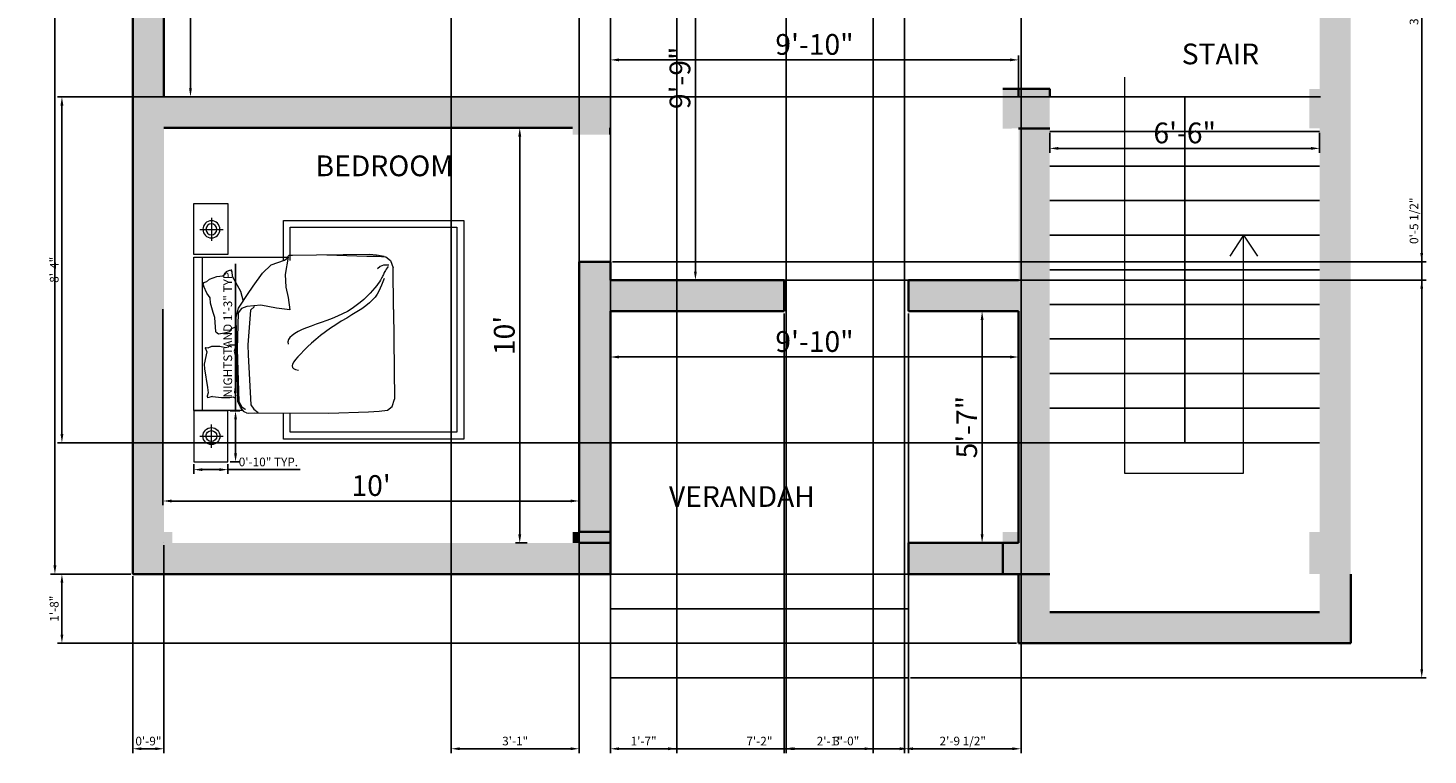
# Model space of a CAD drawing. Units: inches. Extents: x 3025 to 3429, y 1771 to 2198.
# Tile 1 of 3: x 3025 to 3429, y 1771 to 1981. Entities that reach past the tile are written whole.
import ezdxf

# ---------------------------------------------------------------- set-up
doc = ezdxf.new("R2010")
doc.units = ezdxf.units.IN
for name, color, linetype, lineweight in [('A-ANNO-DIMS', 2, 'Continuous', 18), ('A-ANNO-SYMB', 7, 'Continuous', 18), ('A-AREA-IDEN', 7, 'Continuous', 25), ('A-COLS', 7, 'Continuous', 35), ('A-FLOR-STRS', 7, 'Continuous', 25), ('A-FURN', 8, 'Continuous', 18), ('A-WALL', 7, 'Continuous', 35), ('A-WALL-PATT', 3, 'Continuous', 13)]:
    doc.layers.add(name, color=color, linetype=linetype, lineweight=lineweight)
doc.layers.add('A-COLS-PATT', color=18, linetype='Continuous', lineweight=13, true_color=0x000000)
doc.styles.get("Standard").update_dxf_attribs({"font": 'arial.ttf'})
doc.dimstyles.new('ISO-25', dxfattribs={"dimtxt": 2.5, "dimasz": 2.5, "dimexe": 1.25, "dimexo": 0.625, "dimtad": 1, "dimdec": 0, "dimlunit": 3, "dimtxsty": 'Standard', "dimcen": 2.5, "dimadec": 0, "dimazin": 0, "dimtfac": 1, "dimtdec": 0, "dimtmove": 0, "dimatfit": 3, "dimfxl": 1, "dimarcsym": 0})

# ---------------------------------------------------------------- blocks, each defined once
blk = doc.blocks.new('*D2')
at = {"layer": 'A-ANNO-DIMS', "color": 0, "lineweight": -2, "transparency": 16777216}
for p, q in [((3071.28, 2025.21), (3072.84, 2025.21)), ((3071.59, 2022.71), (3071.59, 1963.71)), ((3071.28, 1961.21), (3072.84, 1961.21))]:
    blk.add_line(p, q, dxfattribs=at)
at = {"layer": 'A-ANNO-DIMS', "color": 0, "transparency": 16777216}
for points in [[(3071.17, 2022.71), (3072, 2022.71), (3071.59, 2025.21)], [(3071.17, 1963.71), (3072, 1963.71), (3071.59, 1961.21)]]:
    blk.add_solid(points, dxfattribs=at)
at = {"layer": 'Defpoints', "color": 0, "transparency": 16777216}
for p in [(3070.66, 2025.21), (3070.66, 1961.21), (3071.59, 1961.21)]:
    blk.add_point(p, dxfattribs=at)
at = {"layer": 'A-ANNO-DIMS', "color": 0, "transparency": 16777216, "insert": (3067.91, 1993.21), "char_height": 6, "attachment_point": 5, "rotation": 90}
blk.add_mtext('5\'-4"', dxfattribs=at)
blk = doc.blocks.new('*D4')
at = {"layer": 'A-ANNO-DIMS', "color": 0, "lineweight": -2, "transparency": 16777216}
for p, q in [((3166.97, 1952.21), (3168, 1952.21)), ((3166.75, 1949.71), (3166.75, 1834.71)), ((3168.93, 1832.21), (3165.5, 1832.21))]:
    blk.add_line(p, q, dxfattribs=at)
at = {"layer": 'A-ANNO-DIMS', "color": 0, "transparency": 16777216}
for points in [[(3166.33, 1949.71), (3167.17, 1949.71), (3166.75, 1952.21)], [(3166.33, 1834.71), (3167.17, 1834.71), (3166.75, 1832.21)]]:
    blk.add_solid(points, dxfattribs=at)
at = {"layer": 'Defpoints', "color": 0, "transparency": 16777216}
for p in [(3166.35, 1952.21), (3166.75, 1832.21), (3169.56, 1832.21)]:
    blk.add_point(p, dxfattribs=at)
at = {"layer": 'A-ANNO-DIMS', "color": 0, "transparency": 16777216, "insert": (3163.06, 1892.21), "char_height": 6, "attachment_point": 5, "rotation": 90}
blk.add_mtext("10'", dxfattribs=at)
blk = doc.blocks.new('*D5')
at = {"layer": 'A-ANNO-DIMS', "color": 0, "lineweight": -2, "transparency": 16777216}
for p, q in [((3305.7, 1899.21), (3299.12, 1899.21)), ((3300.37, 1896.71), (3300.37, 1834.71)), ((3305.7, 1832.21), (3299.12, 1832.21))]:
    blk.add_line(p, q, dxfattribs=at)
at = {"layer": 'A-ANNO-DIMS', "color": 0, "transparency": 16777216}
for points in [[(3299.96, 1896.71), (3300.79, 1896.71), (3300.37, 1899.21)], [(3299.96, 1834.71), (3300.79, 1834.71), (3300.37, 1832.21)]]:
    blk.add_solid(points, dxfattribs=at)
at = {"layer": 'Defpoints', "color": 0, "transparency": 16777216}
for p in [(3306.32, 1899.21), (3300.37, 1832.21), (3306.32, 1832.21)]:
    blk.add_point(p, dxfattribs=at)
at = {"layer": 'A-ANNO-DIMS', "color": 0, "transparency": 16777216, "insert": (3296.7, 1865.71), "char_height": 6, "attachment_point": 5, "rotation": 90}
blk.add_mtext('5\'-7"', dxfattribs=at)
blk = doc.blocks.new('*D11')
at = {"layer": 'A-ANNO-DIMS', "color": 0, "lineweight": -2, "transparency": 16777216}
for p, q in [((3192.93, 1961.84), (3192.93, 1973.15)), ((3195.43, 1971.9), (3308.43, 1971.9)), ((3310.93, 1961.84), (3310.93, 1973.15))]:
    blk.add_line(p, q, dxfattribs=at)
at = {"layer": 'A-ANNO-DIMS', "color": 0, "transparency": 16777216}
for points in [[(3195.43, 1972.32), (3195.43, 1971.49), (3192.93, 1971.9)], [(3308.43, 1972.32), (3308.43, 1971.49), (3310.93, 1971.9)]]:
    blk.add_solid(points, dxfattribs=at)
at = {"layer": 'Defpoints', "color": 0, "transparency": 16777216}
for p in [(3310.93, 1971.9), (3192.93, 1961.21), (3310.93, 1961.21)]:
    blk.add_point(p, dxfattribs=at)
at = {"layer": 'A-ANNO-DIMS', "color": 0, "transparency": 16777216, "insert": (3251.93, 1975.59), "char_height": 6, "attachment_point": 5}
blk.add_mtext('9\'-10"', dxfattribs=at)
blk = doc.blocks.new('*D12')
at = {"layer": 'A-ANNO-DIMS', "color": 0, "lineweight": -2, "transparency": 16777216}
for p, q in [((3054.31, 2180.21), (3031.16, 2180.21)), ((3032.41, 2177.71), (3032.41, 1825.71)), ((3054.31, 1823.21), (3031.16, 1823.21))]:
    blk.add_line(p, q, dxfattribs=at)
at = {"layer": 'A-ANNO-DIMS', "color": 0, "transparency": 16777216}
for points in [[(3031.99, 2177.71), (3032.82, 2177.71), (3032.41, 2180.21)], [(3031.99, 1825.71), (3032.82, 1825.71), (3032.41, 1823.21)]]:
    blk.add_solid(points, dxfattribs=at)
at = {"layer": 'Defpoints', "color": 0, "transparency": 16777216}
for p in [(3054.93, 2180.21), (3032.41, 1823.21), (3054.93, 1823.21)]:
    blk.add_point(p, dxfattribs=at)
at = {"layer": 'A-ANNO-DIMS', "color": 0, "transparency": 16777216, "insert": (3028.72, 2001.71), "char_height": 6, "attachment_point": 5, "rotation": 90}
blk.add_mtext('29\'-9"', dxfattribs=at)
blk = doc.blocks.new('*D16')
at = {"layer": 'A-ANNO-DIMS', "color": 0, "lineweight": -2, "transparency": 16777216}
for p, q in [((3319.93, 1950.78), (3319.93, 1945.06)), ((3397.93, 1950.78), (3397.93, 1945.06)), ((3322.43, 1946.31), (3395.43, 1946.31))]:
    blk.add_line(p, q, dxfattribs=at)
at = {"layer": 'A-ANNO-DIMS', "color": 0, "transparency": 16777216}
for points in [[(3322.43, 1946.73), (3322.43, 1945.89), (3319.93, 1946.31)], [(3395.43, 1946.73), (3395.43, 1945.89), (3397.93, 1946.31)]]:
    blk.add_solid(points, dxfattribs=at)
at = {"layer": 'Defpoints', "color": 0, "transparency": 16777216}
for p in [(3319.93, 1951.41), (3397.93, 1951.41), (3397.93, 1946.31)]:
    blk.add_point(p, dxfattribs=at)
at = {"layer": 'A-ANNO-DIMS', "color": 0, "transparency": 16777216, "insert": (3358.93, 1950), "char_height": 6, "attachment_point": 5}
blk.add_mtext('6\'-6"', dxfattribs=at)
blk = doc.blocks.new('*D17')
at = {"layer": 'A-ANNO-DIMS', "color": 0, "lineweight": -2, "transparency": 16777216}
for p, q in [((3225.75, 2025.21), (3216.27, 2025.21)), ((3217.52, 2022.71), (3217.52, 1910.71)), ((3225.75, 1908.21), (3216.27, 1908.21))]:
    blk.add_line(p, q, dxfattribs=at)
at = {"layer": 'A-ANNO-DIMS', "color": 0, "transparency": 16777216}
for points in [[(3217.1, 2022.71), (3217.94, 2022.71), (3217.52, 2025.21)], [(3217.1, 1910.71), (3217.94, 1910.71), (3217.52, 1908.21)]]:
    blk.add_solid(points, dxfattribs=at)
at = {"layer": 'Defpoints', "color": 0, "transparency": 16777216}
for p in [(3226.37, 2025.21), (3217.52, 1908.21), (3226.37, 1908.21)]:
    blk.add_point(p, dxfattribs=at)
at = {"layer": 'A-ANNO-DIMS', "color": 0, "transparency": 16777216, "insert": (3213.83, 1966.71), "char_height": 6, "attachment_point": 5, "rotation": 90}
blk.add_mtext('9\'-9"', dxfattribs=at)
blk = doc.blocks.new('*D18')
at = {"layer": 'A-ANNO-DIMS', "color": 0, "lineweight": -2, "transparency": 16777216}
for p, q in [((3192.93, 1865.6), (3192.93, 1887.24)), ((3195.43, 1885.99), (3308.43, 1885.99)), ((3310.93, 1865.6), (3310.93, 1887.24))]:
    blk.add_line(p, q, dxfattribs=at)
at = {"layer": 'A-ANNO-DIMS', "color": 0, "transparency": 16777216}
for points in [[(3195.43, 1886.4), (3195.43, 1885.57), (3192.93, 1885.99)], [(3308.43, 1886.4), (3308.43, 1885.57), (3310.93, 1885.99)]]:
    blk.add_solid(points, dxfattribs=at)
at = {"layer": 'Defpoints', "color": 0, "transparency": 16777216}
for p in [(3310.93, 1885.99), (3192.93, 1864.97), (3310.93, 1864.97)]:
    blk.add_point(p, dxfattribs=at)
at = {"layer": 'A-ANNO-DIMS', "color": 0, "transparency": 16777216, "insert": (3251.93, 1889.68), "char_height": 6, "attachment_point": 5}
blk.add_mtext('9\'-10"', dxfattribs=at)
blk = doc.blocks.new('*D19')
at = {"layer": 'A-ANNO-DIMS', "color": 0, "lineweight": -2, "transparency": 16777216}
for p, q in [((3063.64, 1899.86), (3063.64, 1843.1)), ((3183.93, 1899.86), (3183.93, 1843.1)), ((3181.43, 1844.35), (3066.14, 1844.35))]:
    blk.add_line(p, q, dxfattribs=at)
at = {"layer": 'A-ANNO-DIMS', "color": 0, "transparency": 16777216}
for points in [[(3066.14, 1844.77), (3066.14, 1843.94), (3063.64, 1844.35)], [(3181.43, 1844.77), (3181.43, 1843.94), (3183.93, 1844.35)]]:
    blk.add_solid(points, dxfattribs=at)
at = {"layer": 'Defpoints', "color": 0, "transparency": 16777216}
for p in [(3063.64, 1900.48), (3183.93, 1900.48), (3063.64, 1844.35)]:
    blk.add_point(p, dxfattribs=at)
at = {"layer": 'A-ANNO-DIMS', "color": 0, "transparency": 16777216, "insert": (3123.79, 1848.04), "char_height": 6, "attachment_point": 5}
blk.add_mtext("10'", dxfattribs=at)
blk = doc.blocks.new('NIGHTSTAND-15IN')
for p, q in [((5.1, 4.12), (5.1, 10.82)), ((1.74, 7.47), (8.45, 7.47))]:
    blk.add_line(p, q)
blk.add_lwpolyline([(9.86, 0), (9.86, 14.79), (0, 14.79), (0, 0)], close=True)
for radius in [2.47, 1.58]:
    blk.add_circle((5.1, 7.47), radius)
blk = doc.blocks.new('*D27')
at = {"layer": 'A-ANNO-DIMS', "color": 0, "lineweight": -2, "transparency": 16777216}
for p, q in [((3084.61, 1870.42), (3084.61, 1912.96)), ((3083.02, 1870.42), (3085.86, 1870.42)), ((3084.61, 1858.14), (3084.61, 1867.92)), ((3083.02, 1855.64), (3085.86, 1855.64))]:
    blk.add_line(p, q, dxfattribs=at)
at = {"layer": 'A-ANNO-DIMS', "color": 0, "transparency": 16777216}
for points in [[(3084.2, 1867.92), (3085.03, 1867.92), (3084.61, 1870.42)], [(3084.2, 1858.14), (3085.03, 1858.14), (3084.61, 1855.64)]]:
    blk.add_solid(points, dxfattribs=at)
at = {"layer": 'Defpoints', "color": 0, "transparency": 16777216}
for p in [(3082.39, 1870.42), (3084.61, 1870.42), (3082.39, 1855.64)]:
    blk.add_point(p, dxfattribs=at)
at = {"layer": 'A-ANNO-DIMS', "color": 0, "transparency": 16777216, "insert": (3082.69, 1892.94), "char_height": 2.5, "attachment_point": 5, "rotation": 90}
blk.add_mtext('NIGHTSTAND 1\'-3" TYP.', dxfattribs=at)
blk = doc.blocks.new('*D28')
at = {"layer": 'A-ANNO-DIMS', "color": 0, "lineweight": -2, "transparency": 16777216}
for p, q in [((3072.54, 1855.01), (3072.54, 1852.17)), ((3075.04, 1853.42), (3079.89, 1853.42)), ((3082.39, 1855.01), (3082.39, 1852.17)), ((3082.39, 1853.42), (3103.33, 1853.42))]:
    blk.add_line(p, q, dxfattribs=at)
at = {"layer": 'A-ANNO-DIMS', "color": 0, "transparency": 16777216}
for points in [[(3075.04, 1853.84), (3075.04, 1853), (3072.54, 1853.42)], [(3079.89, 1853.84), (3079.89, 1853), (3082.39, 1853.42)]]:
    blk.add_solid(points, dxfattribs=at)
at = {"layer": 'Defpoints', "color": 0, "transparency": 16777216}
for p in [(3072.54, 1855.64), (3082.39, 1855.64), (3082.39, 1853.42)]:
    blk.add_point(p, dxfattribs=at)
at = {"layer": 'A-ANNO-DIMS', "color": 0, "transparency": 16777216, "insert": (3094.11, 1855.32), "char_height": 2.5, "attachment_point": 5}
blk.add_mtext('0\'-10" TYP.', dxfattribs=at)
blk = doc.blocks.new('*D29')
at = {"layer": 'A-ANNO-DIMS', "color": 0, "lineweight": -2, "transparency": 16777216}
for p, q in [((3407.56, 2180.21), (3428.68, 2180.21)), ((3427.43, 2177.71), (3427.43, 1795.71)), ((3279.71, 1793.21), (3428.68, 1793.21))]:
    blk.add_line(p, q, dxfattribs=at)
at = {"layer": 'A-ANNO-DIMS', "color": 0, "transparency": 16777216}
for points in [[(3427.02, 2177.71), (3427.85, 2177.71), (3427.43, 2180.21)], [(3427.02, 1795.71), (3427.85, 1795.71), (3427.43, 1793.21)]]:
    blk.add_solid(points, dxfattribs=at)
at = {"layer": 'Defpoints', "color": 0, "transparency": 16777216}
for p in [(3406.93, 2180.21), (3279.09, 1793.21), (3427.43, 1793.21)]:
    blk.add_point(p, dxfattribs=at)
at = {"layer": 'A-ANNO-DIMS', "color": 0, "transparency": 16777216, "insert": (3425.53, 1986.71), "char_height": 2.5, "attachment_point": 5, "rotation": 90}
blk.add_mtext('32\'-3"', dxfattribs=at)
blk = doc.blocks.new('*D30')
at = {"layer": 'A-ANNO-DIMS', "color": 0, "lineweight": -2, "transparency": 16777216}
for p, q in [((3192.93, 1792.59), (3192.93, 1771.46)), ((3279.09, 1792.59), (3279.09, 1771.46)), ((3195.43, 1772.71), (3276.59, 1772.71))]:
    blk.add_line(p, q, dxfattribs=at)
at = {"layer": 'A-ANNO-DIMS', "color": 0, "transparency": 16777216}
for points in [[(3195.43, 1773.13), (3195.43, 1772.3), (3192.93, 1772.71)], [(3276.59, 1773.13), (3276.59, 1772.3), (3279.09, 1772.71)]]:
    blk.add_solid(points, dxfattribs=at)
at = {"layer": 'Defpoints', "color": 0, "transparency": 16777216}
for p in [(3192.93, 1793.21), (3279.09, 1793.21), (3279.09, 1772.71)]:
    blk.add_point(p, dxfattribs=at)
at = {"layer": 'A-ANNO-DIMS', "color": 0, "transparency": 16777216, "insert": (3236.01, 1774.59), "char_height": 2.5, "attachment_point": 5}
blk.add_mtext('7\'-2"', dxfattribs=at)
blk = doc.blocks.new('*D31')
at = {"layer": 'A-ANNO-DIMS', "color": 0, "lineweight": -2, "transparency": 16777216}
for p, q in [((3243.14, 1898.59), (3243.14, 1771.46)), ((3279.09, 1898.59), (3279.09, 1771.46)), ((3245.64, 1772.71), (3276.59, 1772.71))]:
    blk.add_line(p, q, dxfattribs=at)
at = {"layer": 'A-ANNO-DIMS', "color": 0, "transparency": 16777216}
for points in [[(3245.64, 1773.13), (3245.64, 1772.3), (3243.14, 1772.71)], [(3276.59, 1773.13), (3276.59, 1772.3), (3279.09, 1772.71)]]:
    blk.add_solid(points, dxfattribs=at)
at = {"layer": 'Defpoints', "color": 0, "transparency": 16777216}
for p in [(3243.14, 1899.21), (3279.09, 1899.21), (3279.09, 1772.71)]:
    blk.add_point(p, dxfattribs=at)
at = {"layer": 'A-ANNO-DIMS', "color": 0, "transparency": 16777216, "insert": (3261.11, 1774.62), "char_height": 2.5, "attachment_point": 5}
blk.add_mtext('3\'-0"', dxfattribs=at)
blk = doc.blocks.new('*D32')
at = {"layer": 'A-ANNO-DIMS', "color": 0, "lineweight": -2, "transparency": 16777216}
for p, q in [((3063.93, 1831.59), (3063.93, 1771.46)), ((3054.93, 1822.59), (3054.93, 1771.46)), ((3057.43, 1772.71), (3061.43, 1772.71))]:
    blk.add_line(p, q, dxfattribs=at)
at = {"layer": 'A-ANNO-DIMS', "color": 0, "transparency": 16777216}
for points in [[(3057.43, 1773.13), (3057.43, 1772.3), (3054.93, 1772.71)], [(3061.43, 1773.13), (3061.43, 1772.3), (3063.93, 1772.71)]]:
    blk.add_solid(points, dxfattribs=at)
at = {"layer": 'Defpoints', "color": 0, "transparency": 16777216}
for p in [(3063.93, 1832.21), (3054.93, 1823.21), (3063.93, 1772.71)]:
    blk.add_point(p, dxfattribs=at)
at = {"layer": 'A-ANNO-DIMS', "color": 0, "transparency": 16777216, "insert": (3059.43, 1774.61), "char_height": 2.5, "attachment_point": 5}
blk.add_mtext('0\'-9"', dxfattribs=at)
blk = doc.blocks.new('*D33')
at = {"layer": 'A-ANNO-DIMS', "color": 0, "lineweight": -2, "transparency": 16777216}
for p, q in [((3054.31, 1823.21), (3033.18, 1823.21)), ((3034.43, 1820.71), (3034.43, 1805.71)), ((3310.31, 1803.21), (3033.18, 1803.21))]:
    blk.add_line(p, q, dxfattribs=at)
at = {"layer": 'A-ANNO-DIMS', "color": 0, "transparency": 16777216}
for points in [[(3034.02, 1820.71), (3034.85, 1820.71), (3034.43, 1823.21)], [(3034.02, 1805.71), (3034.85, 1805.71), (3034.43, 1803.21)]]:
    blk.add_solid(points, dxfattribs=at)
at = {"layer": 'Defpoints', "color": 0, "transparency": 16777216}
for p in [(3054.93, 1823.21), (3034.43, 1803.21), (3310.93, 1803.21)]:
    blk.add_point(p, dxfattribs=at)
at = {"layer": 'A-ANNO-DIMS', "color": 0, "transparency": 16777216, "insert": (3032.53, 1813.21), "char_height": 2.5, "attachment_point": 5, "rotation": 90}
blk.add_mtext('1\'-8"', dxfattribs=at)
blk = doc.blocks.new('*D34')
at = {"layer": 'A-ANNO-DIMS', "color": 0, "lineweight": -2, "transparency": 16777216}
for p, q in [((3358.31, 1961.21), (3033.18, 1961.21)), ((3034.43, 1958.71), (3034.43, 1863.71)), ((3358.31, 1861.21), (3033.18, 1861.21))]:
    blk.add_line(p, q, dxfattribs=at)
at = {"layer": 'A-ANNO-DIMS', "color": 0, "transparency": 16777216}
for points in [[(3034.02, 1958.71), (3034.85, 1958.71), (3034.43, 1961.21)], [(3034.02, 1863.71), (3034.85, 1863.71), (3034.43, 1861.21)]]:
    blk.add_solid(points, dxfattribs=at)
at = {"layer": 'Defpoints', "color": 0, "transparency": 16777216}
for p in [(3358.93, 1961.21), (3034.43, 1861.21), (3358.93, 1861.21)]:
    blk.add_point(p, dxfattribs=at)
at = {"layer": 'A-ANNO-DIMS', "color": 0, "transparency": 16777216, "insert": (3032.53, 1911.21), "char_height": 2.5, "attachment_point": 5, "rotation": 90}
blk.add_mtext('8\'-4"', dxfattribs=at)
blk = doc.blocks.new('*D35')
at = {"layer": 'A-ANNO-DIMS', "color": 0, "lineweight": -2, "transparency": 16777216}
for p, q in [((3268.93, 2036.1), (3268.93, 1771.46)), ((3243.74, 2033.59), (3243.74, 1771.46)), ((3246.24, 1772.71), (3266.43, 1772.71))]:
    blk.add_line(p, q, dxfattribs=at)
at = {"layer": 'A-ANNO-DIMS', "color": 0, "transparency": 16777216}
for points in [[(3246.24, 1773.13), (3246.24, 1772.3), (3243.74, 1772.71)], [(3266.43, 1773.13), (3266.43, 1772.3), (3268.93, 1772.71)]]:
    blk.add_solid(points, dxfattribs=at)
at = {"layer": 'Defpoints', "color": 0, "transparency": 16777216}
for p in [(3268.93, 2036.73), (3243.74, 2034.21), (3268.93, 1772.71)]:
    blk.add_point(p, dxfattribs=at)
at = {"layer": 'A-ANNO-DIMS', "color": 0, "transparency": 16777216, "insert": (3256.34, 1774.59), "char_height": 2.5, "attachment_point": 5}
blk.add_mtext('2\'-1"', dxfattribs=at)
blk = doc.blocks.new('*D36')
at = {"layer": 'A-ANNO-DIMS', "color": 0, "lineweight": -2, "transparency": 16777216}
for p, q in [((3277.93, 2036.1), (3277.93, 1771.46)), ((3311.62, 2033.59), (3311.62, 1771.46)), ((3280.43, 1772.71), (3309.12, 1772.71))]:
    blk.add_line(p, q, dxfattribs=at)
at = {"layer": 'A-ANNO-DIMS', "color": 0, "transparency": 16777216}
for points in [[(3280.43, 1773.13), (3280.43, 1772.3), (3277.93, 1772.71)], [(3309.12, 1773.13), (3309.12, 1772.3), (3311.62, 1772.71)]]:
    blk.add_solid(points, dxfattribs=at)
at = {"layer": 'Defpoints', "color": 0, "transparency": 16777216}
for p in [(3277.93, 2036.73), (3311.62, 2034.21), (3311.62, 1772.71)]:
    blk.add_point(p, dxfattribs=at)
at = {"layer": 'A-ANNO-DIMS', "color": 0, "transparency": 16777216, "insert": (3294.78, 1774.63), "char_height": 2.5, "attachment_point": 5}
blk.add_mtext('2\'-9 1/2"', dxfattribs=at)
blk = doc.blocks.new('*D37')
at = {"layer": 'A-ANNO-DIMS', "color": 0, "lineweight": -2, "transparency": 16777216}
for p, q in [((3183.93, 2035.84), (3183.93, 1771.46)), ((3146.93, 2033.59), (3146.93, 1771.46)), ((3149.43, 1772.71), (3181.43, 1772.71))]:
    blk.add_line(p, q, dxfattribs=at)
at = {"layer": 'A-ANNO-DIMS', "color": 0, "transparency": 16777216}
for points in [[(3149.43, 1773.13), (3149.43, 1772.3), (3146.93, 1772.71)], [(3181.43, 1773.13), (3181.43, 1772.3), (3183.93, 1772.71)]]:
    blk.add_solid(points, dxfattribs=at)
at = {"layer": 'Defpoints', "color": 0, "transparency": 16777216}
for p in [(3183.93, 2036.47), (3146.93, 2034.21), (3183.93, 1772.71)]:
    blk.add_point(p, dxfattribs=at)
at = {"layer": 'A-ANNO-DIMS', "color": 0, "transparency": 16777216, "insert": (3165.43, 1774.62), "char_height": 2.5, "attachment_point": 5}
blk.add_mtext('3\'-1"', dxfattribs=at)
blk = doc.blocks.new('*D38')
at = {"layer": 'A-ANNO-DIMS', "color": 0, "lineweight": -2, "transparency": 16777216}
for p, q in [((3427.43, 1916.03), (3427.43, 1932.25)), ((3193.56, 1913.53), (3428.68, 1913.53)), ((3427.43, 1908.21), (3427.43, 1913.53)), ((3193.56, 1908.21), (3428.68, 1908.21)), ((3427.43, 1905.71), (3427.43, 1903.21))]:
    blk.add_line(p, q, dxfattribs=at)
at = {"layer": 'A-ANNO-DIMS', "color": 0, "transparency": 16777216}
for points in [[(3427.02, 1916.03), (3427.85, 1916.03), (3427.43, 1913.53)], [(3427.02, 1905.71), (3427.85, 1905.71), (3427.43, 1908.21)]]:
    blk.add_solid(points, dxfattribs=at)
at = {"layer": 'Defpoints', "color": 0, "transparency": 16777216}
for p in [(3192.93, 1913.53), (3427.43, 1913.53), (3192.93, 1908.21)]:
    blk.add_point(p, dxfattribs=at)
at = {"layer": 'A-ANNO-DIMS', "color": 0, "transparency": 16777216, "insert": (3425.52, 1925.39), "char_height": 2.5, "attachment_point": 5, "rotation": 90}
blk.add_mtext('0\'-5 1/2"', dxfattribs=at)
blk = doc.blocks.new('*D40')
at = {"layer": 'A-ANNO-DIMS', "color": 0, "lineweight": -2, "transparency": 16777216}
for p, q in [((3192.93, 2033.59), (3192.93, 1771.46)), ((3212.14, 2033.59), (3212.14, 1771.46)), ((3195.43, 1772.71), (3209.64, 1772.71))]:
    blk.add_line(p, q, dxfattribs=at)
at = {"layer": 'A-ANNO-DIMS', "color": 0, "transparency": 16777216}
for points in [[(3195.43, 1773.13), (3195.43, 1772.3), (3192.93, 1772.71)], [(3209.64, 1773.13), (3209.64, 1772.3), (3212.14, 1772.71)]]:
    blk.add_solid(points, dxfattribs=at)
at = {"layer": 'Defpoints', "color": 0, "transparency": 16777216}
for p in [(3192.93, 2034.21), (3212.14, 2034.21), (3212.14, 1772.71)]:
    blk.add_point(p, dxfattribs=at)
at = {"layer": 'A-ANNO-DIMS', "color": 0, "transparency": 16777216, "insert": (3202.54, 1774.59), "char_height": 2.5, "attachment_point": 5}
blk.add_mtext('1\'-7"', dxfattribs=at)

msp = doc.modelspace()

# ---------------------------------------------------------------- hatches: boundary and pattern name
at = {"layer": 'A-COLS-PATT'}
h = msp.add_hatch(color=256, dxfattribs=at)
h.dxf.hatch_style = 1
h.paths.add_polyline_path([(3310.93, 1835.41), (3306.32, 1835.41), (3306.32, 1832.21), (3310.93, 1832.21)], flags=17)
h.paths.add_polyline_path([(3319.93, 1832.21), (3319.93, 1835.41), (3310.93, 1835.41), (3310.93, 1832.21), (3306.32, 1832.21), (3306.32, 1823.21), (3310.93, 1823.21), (3319.93, 1823.21)])
h.paths.add_polyline_path([(3310.93, 1961.21), (3310.93, 1963.51), (3306.32, 1963.51), (3306.32, 1952.02), (3310.93, 1952.09)])
h.paths.add_polyline_path([(3319.93, 1961.21), (3310.93, 1961.21), (3310.93, 1952.09), (3319.93, 1952.09)])
h = msp.add_hatch(color=256, dxfattribs=at)
h.dxf.hatch_style = 1
h.paths.add_polyline_path([(3397.93, 1963.51), (3394.99, 1963.51), (3394.99, 1961.21), (3397.93, 1961.21)])
h.paths.add_polyline_path([(3319.94, 1963.51), (3310.93, 1963.51), (3310.93, 1961.21), (3319.94, 1961.21)])
h.paths.add_polyline_path([(3397.93, 1961.21), (3394.99, 1961.21), (3394.99, 1952.09), (3397.93, 1952.09)])
h.paths.add_polyline_path([(3406.93, 1963.51), (3397.93, 1963.51), (3397.93, 1952.09), (3406.93, 1952.09)])
h.paths.add_polyline_path([(3397.93, 1832.21), (3397.93, 1835.41), (3394.99, 1835.41), (3394.99, 1823.21), (3397.93, 1823.21)])
h.paths.add_polyline_path([(3406.93, 1835.41), (3397.93, 1835.41), (3397.93, 1832.21), (3397.93, 1823.21), (3406.93, 1823.21)])
h = msp.add_hatch(color=256, dxfattribs=at)
h.dxf.hatch_style = 1
h.paths.add_polyline_path([(3192.93, 1961.21), (3182.07, 1961.21), (3182.07, 1952.21), (3192.93, 1952.21)])
h = msp.add_hatch(color=256, dxfattribs=at)
h.dxf.hatch_style = 1
h.paths.add_polyline_path([(3192.87, 1952.21), (3182.07, 1952.21), (3182.07, 1950.3), (3192.87, 1950.3)])
h = msp.add_hatch(color=256, dxfattribs=at)
h.dxf.hatch_style = 1
h.paths.add_polyline_path([(3066.3, 1832.21), (3063.93, 1832.21), (3063.93, 1835.41), (3054.93, 1835.41), (3054.93, 1823.21), (3066.3, 1823.21)])
h.paths.add_polyline_path([(3066.3, 1835.41), (3063.93, 1835.41), (3063.93, 1832.21), (3066.3, 1832.21)], flags=17)
h = msp.add_hatch(color=256, dxfattribs=at)
h.dxf.hatch_style = 1
h.paths.add_polyline_path([(3183.93, 1835.41), (3182.07, 1835.41), (3182.07, 1832.21), (3183.93, 1832.21)])
h = msp.add_hatch(color=256, dxfattribs=at)
h.dxf.hatch_style = 1
h.paths.add_polyline_path([(3192.93, 1835.41), (3183.93, 1835.41), (3183.93, 1832.21), (3192.93, 1832.21)])
h = msp.add_hatch(color=256, dxfattribs=at)
h.dxf.hatch_style = 1
h.paths.add_polyline_path([(3192.93, 1832.21), (3183.93, 1832.21), (3182.07, 1832.21), (3182.07, 1823.21), (3192.93, 1823.21)])
at = {"layer": 'A-WALL-PATT'}
h = msp.add_hatch(color=256, dxfattribs=at)
h.dxf.hatch_style = 1
h.paths.add_polyline_path([(3063.93, 1952.21), (3192.93, 1952.21), (3192.93, 1961.21), (3063.93, 1961.21), (3063.93, 2025.21), (3054.93, 2025.21), (3054.93, 1823.21), (3192.93, 1823.21), (3192.93, 1832.21), (3183.93, 1832.21), (3063.93, 1832.21)])
h.paths.add_polyline_path([(3146.93, 2034.21), (3063.93, 2034.21), (3063.93, 2036.54), (3054.93, 2036.54), (3054.93, 2025.21), (3063.93, 2025.21), (3137.93, 2025.21), (3137.93, 1993.21), (3146.93, 1993.21)])
h.paths.add_polyline_path([(3063.93, 2167.94), (3054.93, 2167.94), (3054.93, 2036.54), (3063.93, 2036.54)])
h.paths.add_polyline_path([(3182.07, 2180.21), (3066.24, 2180.21), (3066.24, 2171.21), (3182.07, 2171.21)])
h.paths.add_polyline_path([(3192.93, 2114.21), (3243.74, 2114.21), (3243.74, 2123.21), (3192.93, 2123.21), (3192.93, 2167.95), (3183.93, 2167.95), (3183.93, 2036.47), (3192.93, 2036.47)])
h = msp.add_hatch(color=256, dxfattribs=at)
h.dxf.hatch_style = 1
h.paths.add_polyline_path([(3406.93, 1823.21), (3397.93, 1823.21), (3397.93, 1812.21), (3319.93, 1812.21), (3319.93, 1823.21), (3310.93, 1823.21), (3310.93, 1803.21), (3406.93, 1803.21)])
h.paths.add_polyline_path([(3406.93, 1952.09), (3397.93, 1952.09), (3397.93, 1835.41), (3406.93, 1835.41)])
h.paths.add_polyline_path([(3406.93, 2025.21), (3397.93, 2025.21), (3397.93, 1963.51), (3406.93, 1963.51)])
h = msp.add_hatch(color=256, dxfattribs=at)
h.dxf.hatch_style = 1
h.paths.add_polyline_path([(3306.32, 1908.21), (3279.09, 1908.21), (3279.09, 1899.21), (3306.32, 1899.21)])
h.paths.add_polyline_path([(3319.93, 1952.09), (3310.93, 1952.09), (3310.93, 1908.21), (3306.32, 1908.21), (3306.32, 1899.21), (3310.93, 1899.21), (3310.93, 1841.21), (3310.93, 1835.41), (3319.93, 1835.41)])
h = msp.add_hatch(color=256, dxfattribs=at)
h.dxf.hatch_style = 1
h.paths.add_polyline_path([(3243.14, 1899.21), (3243.14, 1908.21), (3192.93, 1908.21), (3192.93, 1913.53), (3183.93, 1913.53), (3183.93, 1835.41), (3192.93, 1835.41), (3192.93, 1899.21)])
h = msp.add_hatch(color=256, dxfattribs=at)
h.dxf.hatch_style = 1
h.paths.add_polyline_path([(3306.32, 1832.21), (3279.09, 1832.21), (3279.09, 1823.21), (3306.32, 1823.21)])

# ---------------------------------------------------------------- linework, layer by layer
at = {"layer": 'A-ANNO-SYMB'}
for p, q in [((3341.52, 1966.91), (3341.52, 1852.41)), ((3375.96, 1921.21), (3371.98, 1915.16)), ((3375.96, 1852.41), (3375.96, 1921.21)), ((3375.96, 1921.21), (3379.95, 1915.16)), ((3341.52, 1852.41), (3375.96, 1852.41))]:
    msp.add_line(p, q, dxfattribs=at)
at = {"layer": 'A-COLS'}
for p, q in [((3306.32, 1963.51), (3310.93, 1963.51)), ((3310.93, 1963.51), (3310.93, 1961.21)), ((3310.93, 1963.51), (3319.94, 1963.51)), ((3319.94, 1963.51), (3319.94, 1961.21)), ((3192.87, 1950.3), (3192.87, 1952.21)), ((3310.93, 1952.09), (3319.93, 1952.09)), ((3183.93, 1835.41), (3192.93, 1835.41)), ((3183.93, 1832.21), (3192.93, 1832.21)), ((3306.32, 1832.21), (3306.32, 1823.21)), ((3310.93, 1823.21), (3319.93, 1823.21))]:
    msp.add_line(p, q, dxfattribs=at)
at = {"layer": 'A-FLOR-STRS'}
for p, q in [((3358.93, 1961.21), (3319.94, 1961.21)), ((3358.93, 1961.21), (3358.93, 1861.21)), ((3358.93, 1961.21), (3398.16, 1961.21)), ((3319.93, 1951.21), (3397.93, 1951.21)), ((3319.93, 1941.21), (3397.93, 1941.21)), ((3319.93, 1931.21), (3397.93, 1931.21)), ((3319.93, 1921.21), (3397.93, 1921.21)), ((3319.93, 1911.21), (3397.93, 1911.21)), ((3319.93, 1901.21), (3397.93, 1901.21)), ((3319.93, 1891.21), (3397.93, 1891.21)), ((3319.93, 1881.21), (3397.93, 1881.21)), ((3319.93, 1871.21), (3397.93, 1871.21)), ((3319.93, 1861.21), (3397.93, 1861.21)), ((3192.93, 1823.21), (3279.09, 1823.21)), ((3192.93, 1823.21), (3192.93, 1813.21)), ((3279.09, 1793.21), (3279.09, 1823.21)), ((3192.93, 1813.21), (3192.93, 1803.21)), ((3192.93, 1813.21), (3279.09, 1813.21)), ((3192.93, 1803.21), (3192.93, 1793.21)), ((3192.93, 1803.21), (3279.09, 1803.21)), ((3192.93, 1793.21), (3279.09, 1793.21))]:
    msp.add_line(p, q, dxfattribs=at)
at = {"layer": 'A-FURN'}
for p, q in [((3099.76, 1914.78), (3099.72, 1914.87)), ((3108.02, 1915.44), (3101.05, 1915.37)), ((3123.28, 1915.59), (3108.02, 1915.44)), ((3111.01, 1915.49), (3122.54, 1915.19)), ((3122.54, 1915.19), (3125.56, 1915.12)), ((3125.39, 1915.47), (3123.28, 1915.59)), ((3127.59, 1915.05), (3125.39, 1915.47)), ((3125.56, 1915.12), (3128.05, 1914.92)), ((3128.05, 1914.92), (3129.39, 1913.88)), ((3129.39, 1913.88), (3130.16, 1911.8)), ((3080.93, 1909.46), (3081.59, 1909.99)), ((3081.59, 1909.99), (3082.02, 1910.68)), ((3082.02, 1910.68), (3083.11, 1911.15)), ((3083.11, 1911.15), (3083.56, 1910.57)), ((3083.56, 1910.57), (3083.61, 1909.37)), ((3126.4, 1912.19), (3125.65, 1911.47)), ((3127.42, 1912.52), (3126.4, 1912.19)), ((3128.88, 1912.59), (3127.42, 1912.52)), ((3130.16, 1906.86), (3130.16, 1911.8)), ((3076.36, 1904.45), (3075.44, 1906.41)), ((3076.21, 1907.74), (3077.07, 1908.52)), ((3077.07, 1908.52), (3079.21, 1909.27)), ((3079.21, 1909.27), (3080.93, 1909.46)), ((3083.61, 1909.37), (3086.06, 1905)), ((3130.3, 1904.99), (3130.16, 1906.86)), ((3077.28, 1903.07), (3076.36, 1904.45)), ((3077.28, 1903.07), (3076.36, 1904.45)), ((3077.41, 1901.51), (3077.28, 1903.07)), ((3130.3, 1899.7), (3130.3, 1904.99)), ((3078.13, 1898.84), (3077.41, 1901.51)), ((3078.66, 1897.43), (3078.13, 1898.84)), ((3130.3, 1899.7), (3130.58, 1873.8)), ((3078.9, 1893.26), (3078.66, 1897.43)), ((3076.28, 1887.52), (3075.52, 1883.89)), ((3075.9, 1888.75), (3075.87, 1888.64)), ((3075.87, 1888.64), (3076.28, 1887.52)), ((3075.9, 1888.75), (3076.72, 1888.66)), ((3075.9, 1888.75), (3076.72, 1888.66)), ((3076.72, 1888.66), (3077.79, 1889.11)), ((3077.79, 1889.11), (3080.06, 1889.09)), ((3080.06, 1889.09), (3081.74, 1888.69)), ((3081.74, 1888.69), (3082.54, 1888.97)), ((3082.54, 1888.97), (3083.18, 1889.46)), ((3083.18, 1889.46), (3084.37, 1889.53)), ((3084.6, 1888.84), (3084.24, 1887.7)), ((3084.24, 1887.7), (3085.15, 1884.1)), ((3084.37, 1889.53), (3084.6, 1888.84)), ((3075.52, 1883.89), (3075.67, 1882.54)), ((3077.96, 1874.56), (3076.53, 1874.18)), ((3129.88, 1871.7), (3130.58, 1873.8)), ((3086.8, 1870.48), (3072.54, 1870.48)), ((3087.78, 1869.85), (3088.47, 1869.79)), ((3088.47, 1869.79), (3090.07, 1869.81)), ((3090.07, 1869.81), (3111.55, 1869.72)), ((3111.55, 1869.72), (3123.06, 1870.18)), ((3123.06, 1870.18), (3126.08, 1870.34)), ((3126.08, 1870.34), (3128.56, 1870.62)), ((3128.56, 1870.62), (3129.88, 1871.7))]:
    msp.add_line(p, q, dxfattribs=at)
for points in [[(3098.46, 1913.9), (3098.46, 1925.5), (3150.56, 1925.5), (3150.56, 1862.24), (3098.46, 1862.24), (3098.46, 1869.78)], [(3100.43, 1913.9), (3100.43, 1923.53), (3148.59, 1923.53), (3148.59, 1864.21), (3100.43, 1864.21), (3100.43, 1869.78)], [(3072.54, 1870.48), (3072.54, 1914.85), (3099.68, 1914.85)], [(3075, 1914.85), (3075, 1870.48)], [(3086.53, 1870.85), (3086, 1871.46), (3085.31, 1873.12), (3084.83, 1897.64), (3085.46, 1900.1), (3088.07, 1904.04), (3089.71, 1906.51), (3092.44, 1910.23), (3094.86, 1912.6), (3098.74, 1914), (3099.75, 1914.69)], [(3099.78, 1914.85), (3098.91, 1909.88), (3099.19, 1906.21), (3099.79, 1903.21), (3100.29, 1899.65), (3096.41, 1900.13), (3091.89, 1900.93), (3087.9, 1900.58), (3086.29, 1900.06), (3085.37, 1898.76), (3085.08, 1888.24), (3085.53, 1873.13), (3086.45, 1871.58), (3087.35, 1870.93), (3087.43, 1870.84)], [(3100.99, 1915.37), (3100.03, 1915.3), (3099.74, 1915.02), (3099.68, 1914.85)], [(3128.72, 1912.15), (3128.41, 1911.74), (3128.15, 1911.37), (3127.94, 1911.03), (3127.76, 1910.71), (3127.61, 1910.41), (3127.48, 1910.13), (3127.35, 1909.84), (3127.22, 1909.56), (3127.09, 1909.26), (3126.93, 1908.94), (3126.74, 1908.59), (3126.5, 1908.2), (3126.2, 1907.75), (3125.84, 1907.24), (3125.4, 1906.67), (3124.86, 1906), (3124.23, 1905.26), (3123.49, 1904.44), (3122.64, 1903.57), (3121.7, 1902.66), (3120.66, 1901.75), (3119.52, 1900.86), (3118.29, 1899.99), (3116.95, 1899.18), (3115.53, 1898.43), (3114.04, 1897.75), (3112.5, 1897.13), (3110.95, 1896.54), (3109.4, 1895.99), (3107.89, 1895.47), (3106.44, 1894.95), (3105.08, 1894.43), (3103.82, 1893.91), (3102.7, 1893.37), (3101.73, 1892.82), (3100.93, 1892.25), (3100.32, 1891.66), (3099.92, 1891.05), (3099.74, 1890.41), (3099.82, 1889.73)], [(3076.21, 1907.74), (3075.31, 1907.46), (3075.12, 1906.87), (3075.44, 1906.41)], [(3127.56, 1908.65), (3127.15, 1907.71), (3126.77, 1906.79), (3126.39, 1905.9), (3125.98, 1905.03), (3125.5, 1904.17), (3124.92, 1903.32), (3124.22, 1902.48), (3123.34, 1901.63), (3122.29, 1900.79), (3121.07, 1899.93), (3119.71, 1899.06), (3118.26, 1898.17), (3116.74, 1897.26), (3115.18, 1896.31), (3113.61, 1895.33), (3112.07, 1894.32), (3110.59, 1893.26), (3109.17, 1892.17), (3107.83, 1891.07), (3106.58, 1889.98), (3105.43, 1888.92), (3104.38, 1887.9), (3103.44, 1886.93), (3102.63, 1886.04), (3101.96, 1885.25), (3101.44, 1884.55), (3101.1, 1883.93), (3100.96, 1883.41), (3101.05, 1882.98), (3101.38, 1882.63), (3101.97, 1882.37), (3102.85, 1882.19)], [(3086.06, 1905), (3086.78, 1902.09)], [(3090.11, 1900.63), (3088.97, 1899.52), (3088.12, 1889.51), (3088.29, 1886.6), (3089.02, 1872.11), (3089.94, 1870.89), (3091.18, 1869.97)], [(3078.9, 1893.26), (3079.72, 1892.69), (3081.44, 1892.96), (3082.94, 1893.38), (3083.42, 1894.2), (3084.66, 1894.68), (3084.88, 1894.68)], [(3075.67, 1882.54), (3076.47, 1877.18), (3076.74, 1875.62), (3076.44, 1874.69), (3076.53, 1874.18)], [(3085.07, 1882.75), (3084.5, 1877.35), (3084.31, 1875.79), (3084.65, 1874.88), (3084.55, 1874.12), (3083.95, 1874.33), (3082.93, 1874.2), (3080.56, 1874.17), (3077.96, 1874.51)], [(3087.73, 1869.87), (3087.27, 1870.02), (3086.92, 1870.23), (3086.8, 1870.48), (3086.54, 1870.77), (3086.53, 1870.81)]]:
    msp.add_lwpolyline(points, dxfattribs=at)
at = {"layer": 'A-WALL'}
for p, q in [((3054.93, 2180.21), (3054.93, 1823.21)), ((3063.93, 2025.21), (3063.93, 1961.21)), ((3063.93, 1952.21), (3182.03, 1952.21)), ((3192.93, 1913.53), (3183.93, 1913.53)), ((3183.93, 1913.53), (3183.93, 1835.41)), ((3192.93, 1913.53), (3192.93, 1908.21)), ((3192.93, 1908.21), (3243.14, 1908.21)), ((3243.14, 1908.21), (3243.14, 1899.21)), ((3279.09, 1908.21), (3279.09, 1899.21)), ((3279.09, 1908.21), (3310.93, 1908.21)), ((3192.93, 1899.21), (3243.14, 1899.21)), ((3192.93, 1899.21), (3192.93, 1823.21)), ((3279.09, 1899.21), (3310.93, 1899.21)), ((3310.93, 1899.21), (3310.93, 1841.21)), ((3310.93, 1841.21), (3310.93, 1832.21)), ((3063.93, 1832.21), (3063.93, 1832.21)), ((3063.93, 1832.21), (3063.93, 1832.21)), ((3279.09, 1832.21), (3279.09, 1823.21)), ((3279.09, 1832.21), (3310.93, 1832.21)), ((3054.93, 1823.21), (3192.93, 1823.21)), ((3279.09, 1823.21), (3310.93, 1823.21)), ((3310.93, 1823.21), (3310.93, 1803.21)), ((3406.93, 1803.21), (3406.93, 1823.21)), ((3319.93, 1812.21), (3397.93, 1812.21)), ((3310.93, 1803.21), (3406.93, 1803.21))]:
    msp.add_line(p, q, dxfattribs=at)

# ---------------------------------------------------------------- block references
at = {"layer": 'A-FURN', "extrusion": (0, 0, -1), "zscale": -1, "rotation": 180}
msp.add_blockref('NIGHTSTAND-15IN', (-3072.54, 1930.37), dxfattribs=at)
at = {"layer": 'A-FURN'}
msp.add_blockref('NIGHTSTAND-15IN', (3072.54, 1855.64), dxfattribs=at)

# ---------------------------------------------------------------- texts
at = {"layer": 'A-AREA-IDEN', "char_height": 6, "attachment_point": 1}
for s, insert in [('STAIR', (3358.07, 1976.62)), ('BEDROOM', (3107.72, 1944.26)), ('VERANDAH', (3209.87, 1848.64))]:
    msp.add_mtext(s, dxfattribs=dict(at, insert=insert))

# ---------------------------------------------------------------- dimensions: what is measured, and where the dimension line sits
at = {"layer": 'A-ANNO-DIMS'}
for base, p1, p2, override, picture, middle in [((3032.41, 1823.21), (3054.93, 2180.21), (3054.93, 1823.21), {"dimtxt": 6, "dimclrd": 0, "dimclre": 0, "dimclrt": 0}, '*D12', (3028.72, 2001.71)), ((3427.43, 1793.21), (3406.93, 2180.21), (3279.09, 1793.21), {"dimdec": 1, "dimlfac": 1, "dimrnd": 0, "dimzin": 1, "dimdsep": 46, "dimlunit": 4, "dimfrac": 2}, '*D29', (3425.53, 1986.71)), ((3071.59, 1961.21), (3070.66, 2025.21), (3070.66, 1961.21), {"dimtxt": 6, "dimclrd": 0, "dimclre": 0, "dimclrt": 0}, '*D2', (3067.91, 1993.21)), ((3217.52, 1908.21), (3226.37, 2025.21), (3226.37, 1908.21), {"dimtxt": 6, "dimclrd": 0, "dimclre": 0, "dimclrt": 0}, '*D17', (3213.83, 1966.71)), ((3034.43, 1861.21), (3358.93, 1961.21), (3358.93, 1861.21), {"dimdec": 1, "dimlfac": 1, "dimrnd": 0, "dimzin": 1, "dimdsep": 46, "dimlunit": 4, "dimfrac": 2}, '*D34', (3032.53, 1911.21)), ((3166.75, 1832.21), (3166.35, 1952.21), (3169.56, 1832.21), {"dimtxt": 6, "dimclrd": 0, "dimclre": 0, "dimclrt": 0}, '*D4', (3163.06, 1892.21)), ((3427.43, 1913.53), (3192.93, 1908.21), (3192.93, 1913.53), {"dimdec": 1, "dimlfac": 1, "dimrnd": 0, "dimzin": 1, "dimdsep": 46, "dimlunit": 4, "dimfrac": 2}, '*D38', (3425.52, 1925.39)), ((3300.37, 1832.21), (3306.32, 1899.21), (3306.32, 1832.21), {"dimtxt": 6, "dimclrd": 0, "dimclre": 0, "dimclrt": 0}, '*D5', (3296.7, 1865.71)), ((3034.43, 1803.21), (3054.93, 1823.21), (3310.93, 1803.21), {"dimdec": 1, "dimlfac": 1, "dimrnd": 0, "dimzin": 1, "dimdsep": 46, "dimlunit": 4, "dimfrac": 2}, '*D33', (3032.53, 1813.21))]:
    dim = msp.add_linear_dim(base=base, p1=p1, p2=p2, angle=90, dimstyle='ISO-25', override=override, dxfattribs=at)
    dim.commit()
    dim.dimension.update_dxf_attribs({"geometry": picture, "text_midpoint": middle})
for base, p1, p2, override, picture, middle in [((3183.93, 1772.71), (3146.93, 2034.21), (3183.93, 2036.47), {"dimdec": 1, "dimlfac": 1, "dimrnd": 0, "dimzin": 1, "dimdsep": 46, "dimlunit": 4, "dimfrac": 2}, '*D37', (3165.43, 1774.62)), ((3268.93, 1772.71), (3243.74, 2034.21), (3268.93, 2036.73), {"dimdec": 1, "dimlfac": 1, "dimrnd": 0, "dimzin": 1, "dimdsep": 46, "dimlunit": 4, "dimfrac": 2}, '*D35', (3256.34, 1774.59)), ((3311.62, 1772.71), (3277.93, 2036.73), (3311.62, 2034.21), {"dimdec": 1, "dimlfac": 1, "dimrnd": 0, "dimzin": 1, "dimdsep": 46, "dimlunit": 4, "dimfrac": 2}, '*D36', (3294.78, 1774.63)), ((3212.14, 1772.71), (3192.93, 2034.21), (3212.14, 2034.21), {"dimdec": 1, "dimlfac": 1, "dimrnd": 0, "dimzin": 1, "dimdsep": 46, "dimlunit": 4, "dimfrac": 2}, '*D40', (3202.54, 1774.59)), ((3310.93, 1971.9), (3192.93, 1961.21), (3310.93, 1961.21), {"dimtxt": 6, "dimclrd": 0, "dimclre": 0, "dimclrt": 0}, '*D11', (3251.93, 1975.59)), ((3397.93, 1946.31), (3319.93, 1951.41), (3397.93, 1951.41), {"dimtxt": 6, "dimclrd": 0, "dimclre": 0, "dimclrt": 0}, '*D16', (3358.93, 1950)), ((3063.64, 1844.35), (3183.93, 1900.48), (3063.64, 1900.48), {"dimtxt": 6, "dimclrd": 0, "dimclre": 0, "dimclrt": 0}, '*D19', (3123.79, 1848.04)), ((3279.0863, 1772.7132), (3243.1428, 1899.2132), (3279.0863, 1899.2132), {"dimdec": 1, "dimlfac": 1, "dimrnd": 0, "dimzin": 1, "dimdsep": 46, "dimlunit": 4, "dimfrac": 2}, '*D31', (3261.1146, 1774.6155)), ((3310.93, 1885.99), (3192.93, 1864.97), (3310.93, 1864.97), {"dimtxt": 6, "dimclrd": 0, "dimclre": 0, "dimclrt": 0}, '*D18', (3251.93, 1889.68)), ((3063.93, 1772.71), (3054.93, 1823.21), (3063.93, 1832.21), {"dimdec": 1, "dimlfac": 1, "dimrnd": 0, "dimzin": 1, "dimdsep": 46, "dimlunit": 4, "dimfrac": 2}, '*D32', (3059.43, 1774.61)), ((3279.09, 1772.71), (3192.93, 1793.21), (3279.09, 1793.21), {"dimdec": 1, "dimlfac": 1, "dimrnd": 0, "dimzin": 1, "dimdsep": 46, "dimlunit": 4, "dimfrac": 2}, '*D30', (3236.01, 1774.59))]:
    dim = msp.add_linear_dim(base=base, p1=p1, p2=p2, dimstyle='ISO-25', override=override, dxfattribs=at)
    dim.commit()
    dim.dimension.update_dxf_attribs({"geometry": picture, "text_midpoint": middle})
dim = msp.add_linear_dim(base=(3084.61, 1870.42), p1=(3082.39, 1855.64), p2=(3082.39, 1870.42), angle=90, text='NIGHTSTAND <> TYP.', dimstyle='ISO-25', override={"dimdec": 1, "dimlfac": 1, "dimrnd": 0, "dimzin": 1, "dimdsep": 46, "dimlunit": 4, "dimfrac": 2}, dxfattribs=at)
dim.commit()
dim.dimension.update_dxf_attribs({"geometry": '*D27', "text_midpoint": (3082.69, 1892.94)})
dim = msp.add_linear_dim(base=(3082.394, 1853.4193), p1=(3072.5373, 1855.637), p2=(3082.394, 1855.637), text='<> TYP.', dimstyle='ISO-25', override={"dimdec": 1, "dimlfac": 1, "dimrnd": 0, "dimzin": 1, "dimdsep": 46, "dimlunit": 4, "dimfrac": 2}, dxfattribs=at)
dim.commit()
dim.dimension.update_dxf_attribs({"geometry": '*D28', "text_midpoint": (3094.1096, 1855.3207)})

doc.saveas('drawing.dxf')
